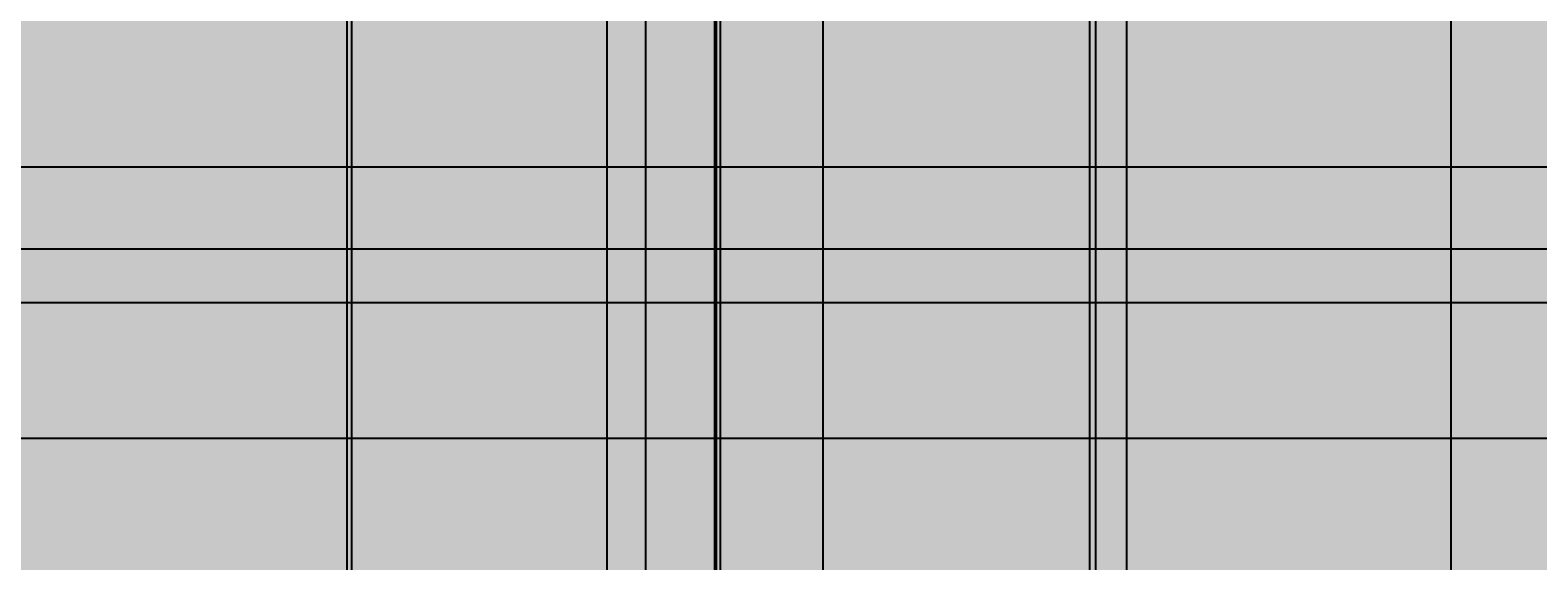
# Model space of a CAD drawing. Units: inches. Extents: x 818 to 1898, y 976 to 2364.
# Tile 75 of 96: x 1260 to 1372, y 2054 to 2093. Entities that reach past the tile are written whole.
import ezdxf

# ---------------------------------------------------------------- set-up
doc = ezdxf.new("R2010")
doc.units = ezdxf.units.IN
doc.header["$LTSCALE"] = 5
doc.header["$MEASUREMENT"] = 0
doc.layers.add('A-ANNO-DIMS', color=2, linetype='Continuous', lineweight=18)
doc.layers.add('L-PLNT-PATT', color=114, linetype='Continuous', lineweight=9, true_color=0x139b48)
doc.styles.get("Standard").update_dxf_attribs({"font": 'arial.ttf'})
doc.dimstyles.get("Standard").update_dxf_attribs({"dimtxt": 0.18, "dimasz": 0.18, "dimexe": 0.18, "dimexo": 0.0625, "dimgap": 0.09, "dimtad": 0, "dimtih": 1, "dimtoh": 1, "dimdec": 4, "dimzin": 0, "dimdsep": 46, "dimtxsty": 'Standard', "dimcen": 0.09, "dimadec": 0, "dimazin": 0, "dimtfac": 1, "dimtdec": 4, "dimtofl": 0, "dimtmove": 0, "dimatfit": 3, "dimfxl": 1, "dimtolj": 1, "dimtzin": 0, "dimarcsym": 0})

# ---------------------------------------------------------------- blocks, each defined once
blk = doc.blocks.new('*D61')
at = {"layer": 'A-ANNO-DIMS', "color": 0, "lineweight": -2, "ltscale": 5, "transparency": 16777216}
for p, q in [((1071.73, 1203.03), (1071.73, 2363.87)), ((1071.91, 2363.69), (1250.94, 2363.69)), ((1430.55, 2363.69), (1251.51, 2363.69)), ((1430.73, 1203.03), (1430.73, 2363.87))]:
    blk.add_line(p, q, dxfattribs=at)
at = {"layer": 'A-ANNO-DIMS', "color": 0, "ltscale": 5, "transparency": 16777216}
for points in [[(1071.91, 2363.72), (1071.91, 2363.66), (1071.73, 2363.69)], [(1430.55, 2363.72), (1430.55, 2363.66), (1430.73, 2363.69)]]:
    blk.add_solid(points, dxfattribs=at)
at = {"layer": 'Defpoints', "color": 0, "ltscale": 5, "transparency": 16777216}
for p in [(1430.73, 2363.69), (1071.73, 1202.96), (1430.73, 1202.96)]:
    blk.add_point(p, dxfattribs=at)
at = {"layer": 'A-ANNO-DIMS', "color": 0, "ltscale": 5, "transparency": 16777216, "insert": (1251.23, 2363.69), "char_height": 0.18, "attachment_point": 5}
blk.add_mtext('\\A1;359', dxfattribs=at)
blk = doc.blocks.new('*D64')
at = {"layer": 'A-ANNO-DIMS', "color": 0, "lineweight": -2, "ltscale": 5, "transparency": 16777216}
for p, q in [((1197.73, 1501.14), (1197.73, 2363.87)), ((1197.91, 2363.69), (1313.93, 2363.69)), ((1430.55, 2363.69), (1314.52, 2363.69)), ((1430.73, 1501.14), (1430.73, 2363.87))]:
    blk.add_line(p, q, dxfattribs=at)
at = {"layer": 'A-ANNO-DIMS', "color": 0, "ltscale": 5, "transparency": 16777216}
for points in [[(1197.91, 2363.72), (1197.91, 2363.66), (1197.73, 2363.69)], [(1430.55, 2363.72), (1430.55, 2363.66), (1430.73, 2363.69)]]:
    blk.add_solid(points, dxfattribs=at)
at = {"layer": 'Defpoints', "color": 0, "ltscale": 5, "transparency": 16777216}
for p in [(1430.73, 2363.69), (1197.73, 1501.08), (1430.73, 1501.08)]:
    blk.add_point(p, dxfattribs=at)
at = {"layer": 'A-ANNO-DIMS', "color": 0, "ltscale": 5, "transparency": 16777216, "insert": (1314.23, 2363.69), "char_height": 0.18, "attachment_point": 5}
blk.add_mtext('\\A1;233', dxfattribs=at)
blk = doc.blocks.new('*D86')
at = {"layer": 'A-ANNO-DIMS', "color": 0, "lineweight": -2, "ltscale": 5, "transparency": 16777216}
for p, q in [((1258.73, 2053.14), (1258.73, 2363.87)), ((1258.91, 2363.69), (1486.43, 2363.69)), ((1714.55, 2363.69), (1487.02, 2363.69)), ((1714.73, 2053.14), (1714.73, 2363.87))]:
    blk.add_line(p, q, dxfattribs=at)
at = {"layer": 'A-ANNO-DIMS', "color": 0, "ltscale": 5, "transparency": 16777216}
for points in [[(1258.91, 2363.72), (1258.91, 2363.66), (1258.73, 2363.69)], [(1714.55, 2363.72), (1714.55, 2363.66), (1714.73, 2363.69)]]:
    blk.add_solid(points, dxfattribs=at)
at = {"layer": 'Defpoints', "color": 0, "ltscale": 5, "transparency": 16777216}
for p in [(1714.73, 2363.69), (1258.73, 2053.08), (1714.73, 2053.08)]:
    blk.add_point(p, dxfattribs=at)
at = {"layer": 'A-ANNO-DIMS', "color": 0, "ltscale": 5, "transparency": 16777216, "insert": (1486.73, 2363.69), "char_height": 0.18, "attachment_point": 5}
blk.add_mtext('\\A1;456', dxfattribs=at)
blk = doc.blocks.new('*D96')
at = {"layer": 'A-ANNO-DIMS', "color": 0, "lineweight": -2, "ltscale": 5, "transparency": 16777216}
for p, q in [((1229.65, 1071.12), (1229.65, 2363.87)), ((1229.83, 2363.69), (1256.52, 2363.69)), ((1283.99, 2363.69), (1257.3, 2363.69)), ((1284.17, 1071.12), (1284.17, 2363.87))]:
    blk.add_line(p, q, dxfattribs=at)
at = {"layer": 'A-ANNO-DIMS', "color": 0, "ltscale": 5, "transparency": 16777216}
for points in [[(1229.83, 2363.72), (1229.83, 2363.66), (1229.65, 2363.69)], [(1283.99, 2363.72), (1283.99, 2363.66), (1284.17, 2363.69)]]:
    blk.add_solid(points, dxfattribs=at)
at = {"layer": 'Defpoints', "color": 0, "ltscale": 5, "transparency": 16777216}
for p in [(1284.17, 2363.69), (1229.65, 1071.06), (1284.17, 1071.06)]:
    blk.add_point(p, dxfattribs=at)
at = {"layer": 'A-ANNO-DIMS', "color": 0, "ltscale": 5, "transparency": 16777216, "insert": (1256.91, 2363.69), "char_height": 0.18, "attachment_point": 5}
blk.add_mtext('\\A1;54.52', dxfattribs=at)
blk = doc.blocks.new('*D97')
at = {"layer": 'A-ANNO-DIMS', "color": 0, "lineweight": -2, "ltscale": 5, "transparency": 16777216}
for p, q in [((1284.17, 1071.12), (1284.17, 2363.87)), ((1284.35, 2363.69), (1310.96, 2363.69)), ((1338.36, 2363.69), (1311.75, 2363.69)), ((1338.54, 1071.12), (1338.54, 2363.87))]:
    blk.add_line(p, q, dxfattribs=at)
at = {"layer": 'A-ANNO-DIMS', "color": 0, "ltscale": 5, "transparency": 16777216}
for points in [[(1284.35, 2363.72), (1284.35, 2363.66), (1284.17, 2363.69)], [(1338.36, 2363.72), (1338.36, 2363.66), (1338.54, 2363.69)]]:
    blk.add_solid(points, dxfattribs=at)
at = {"layer": 'Defpoints', "color": 0, "ltscale": 5, "transparency": 16777216}
for p in [(1338.54, 2363.69), (1284.17, 1071.06), (1338.54, 1071.06)]:
    blk.add_point(p, dxfattribs=at)
at = {"layer": 'A-ANNO-DIMS', "color": 0, "ltscale": 5, "transparency": 16777216, "insert": (1311.36, 2363.69), "char_height": 0.18, "attachment_point": 5}
blk.add_mtext('\\A1;54.37', dxfattribs=at)
blk = doc.blocks.new('*D98')
at = {"layer": 'A-ANNO-DIMS', "color": 0, "lineweight": -2, "ltscale": 5, "transparency": 16777216}
for p, q in [((1338.54, 1071.12), (1338.54, 2363.87)), ((1338.72, 2363.69), (1364.81, 2363.69)), ((1391.7, 2363.69), (1365.6, 2363.69)), ((1391.88, 1071.12), (1391.88, 2363.87))]:
    blk.add_line(p, q, dxfattribs=at)
at = {"layer": 'A-ANNO-DIMS', "color": 0, "ltscale": 5, "transparency": 16777216}
for points in [[(1338.72, 2363.72), (1338.72, 2363.66), (1338.54, 2363.69)], [(1391.7, 2363.72), (1391.7, 2363.66), (1391.88, 2363.69)]]:
    blk.add_solid(points, dxfattribs=at)
at = {"layer": 'Defpoints', "color": 0, "ltscale": 5, "transparency": 16777216}
for p in [(1391.88, 2363.69), (1338.54, 1071.06), (1391.88, 1071.06)]:
    blk.add_point(p, dxfattribs=at)
at = {"layer": 'A-ANNO-DIMS', "color": 0, "ltscale": 5, "transparency": 16777216, "insert": (1365.21, 2363.69), "char_height": 0.18, "attachment_point": 5}
blk.add_mtext('\\A1;53.33', dxfattribs=at)
blk = doc.blocks.new('*D141')
at = {"layer": 'A-ANNO-DIMS', "color": 0, "lineweight": -2, "ltscale": 5, "transparency": 16777216}
for p, q in [((1218.17, 2083.26), (1897.92, 2083.26)), ((1897.74, 2083.08), (1897.74, 2073.44)), ((1897.74, 2063.44), (1897.74, 2073.08)), ((1198.17, 2063.26), (1897.92, 2063.26))]:
    blk.add_line(p, q, dxfattribs=at)
at = {"layer": 'A-ANNO-DIMS', "color": 0, "ltscale": 5, "transparency": 16777216}
for points in [[(1897.71, 2083.08), (1897.77, 2083.08), (1897.74, 2083.26)], [(1897.71, 2063.44), (1897.77, 2063.44), (1897.74, 2063.26)]]:
    blk.add_solid(points, dxfattribs=at)
at = {"layer": 'Defpoints', "color": 0, "ltscale": 5, "transparency": 16777216}
for p in [(1218.11, 2083.26), (1198.11, 2063.26), (1897.74, 2063.26)]:
    blk.add_point(p, dxfattribs=at)
at = {"layer": 'A-ANNO-DIMS', "color": 0, "ltscale": 5, "transparency": 16777216, "insert": (1897.74, 2073.26), "char_height": 0.18, "attachment_point": 5}
blk.add_mtext('\\A1;20', dxfattribs=at)
blk = doc.blocks.new('*D142')
at = {"layer": 'A-ANNO-DIMS', "color": 0, "lineweight": -2, "ltscale": 5, "transparency": 16777216}
for p, q in [((1208.17, 2073.26), (1897.92, 2073.26)), ((1897.74, 2073.08), (1897.74, 2068.44)), ((1897.74, 2063.44), (1897.74, 2068.08)), ((1198.17, 2063.26), (1897.92, 2063.26))]:
    blk.add_line(p, q, dxfattribs=at)
at = {"layer": 'A-ANNO-DIMS', "color": 0, "ltscale": 5, "transparency": 16777216}
for points in [[(1897.71, 2073.08), (1897.77, 2073.08), (1897.74, 2073.26)], [(1897.71, 2063.44), (1897.77, 2063.44), (1897.74, 2063.26)]]:
    blk.add_solid(points, dxfattribs=at)
at = {"layer": 'Defpoints', "color": 0, "ltscale": 5, "transparency": 16777216}
for p in [(1208.11, 2073.26), (1897.74, 2073.26), (1198.11, 2063.26)]:
    blk.add_point(p, dxfattribs=at)
at = {"layer": 'A-ANNO-DIMS', "color": 0, "ltscale": 5, "transparency": 16777216, "insert": (1897.74, 2068.26), "char_height": 0.18, "attachment_point": 5}
blk.add_mtext('\\A1;10', dxfattribs=at)
blk = doc.blocks.new('*D165')
at = {"layer": 'A-ANNO-DIMS', "color": 0, "lineweight": -2, "ltscale": 5, "transparency": 16777216}
for p, q in [((1283.82, 1510.14), (1283.82, 2363.87)), ((1284, 2363.69), (1324.09, 2363.69)), ((1364.97, 2363.69), (1324.88, 2363.69)), ((1365.15, 1510.14), (1365.15, 2363.87))]:
    blk.add_line(p, q, dxfattribs=at)
at = {"layer": 'A-ANNO-DIMS', "color": 0, "ltscale": 5, "transparency": 16777216}
for points in [[(1284, 2363.72), (1284, 2363.66), (1283.82, 2363.69)], [(1364.97, 2363.72), (1364.97, 2363.66), (1365.15, 2363.69)]]:
    blk.add_solid(points, dxfattribs=at)
at = {"layer": 'Defpoints', "color": 0, "ltscale": 5, "transparency": 16777216}
for p in [(1365.15, 2363.69), (1283.82, 1510.08), (1365.15, 1510.08)]:
    blk.add_point(p, dxfattribs=at)
at = {"layer": 'A-ANNO-DIMS', "color": 0, "ltscale": 5, "transparency": 16777216, "insert": (1324.48, 2363.69), "char_height": 0.18, "attachment_point": 5}
blk.add_mtext('\\A1;81.33', dxfattribs=at)
blk = doc.blocks.new('*D235')
at = {"layer": 'A-ANNO-DIMS', "color": 0, "lineweight": -2, "ltscale": 5, "transparency": 16777216}
for p, q in [((1310.91, 2026.27), (1310.91, 2363.87)), ((1311.09, 2363.69), (1324.48, 2363.69)), ((1338.81, 2363.69), (1325.41, 2363.69)), ((1338.99, 2026.27), (1338.99, 2363.87))]:
    blk.add_line(p, q, dxfattribs=at)
at = {"layer": 'A-ANNO-DIMS', "color": 0, "ltscale": 5, "transparency": 16777216}
for points in [[(1311.09, 2363.72), (1311.09, 2363.66), (1310.91, 2363.69)], [(1338.81, 2363.72), (1338.81, 2363.66), (1338.99, 2363.69)]]:
    blk.add_solid(points, dxfattribs=at)
at = {"layer": 'Defpoints', "color": 0, "ltscale": 5, "transparency": 16777216}
for p in [(1338.99, 2363.69), (1310.91, 2026.21), (1338.99, 2026.21)]:
    blk.add_point(p, dxfattribs=at)
at = {"layer": 'A-ANNO-DIMS', "color": 0, "ltscale": 5, "transparency": 16777216, "insert": (1324.95, 2363.69), "char_height": 0.18, "attachment_point": 5}
blk.add_mtext('\\A1;28.084', dxfattribs=at)
blk = doc.blocks.new('*D257')
at = {"layer": 'A-ANNO-DIMS', "color": 0, "lineweight": -2, "ltscale": 5, "transparency": 16777216}
for p, q in [((1399.57, 2077.19), (818.03, 2077.19)), ((818.21, 2077.01), (818.21, 2065.31)), ((818.21, 2053.26), (818.21, 2064.95)), ((1399.57, 2053.08), (818.03, 2053.08))]:
    blk.add_line(p, q, dxfattribs=at)
at = {"layer": 'A-ANNO-DIMS', "color": 0, "ltscale": 5, "transparency": 16777216}
for points in [[(818.18, 2077.01), (818.24, 2077.01), (818.21, 2077.19)], [(818.18, 2053.26), (818.24, 2053.26), (818.21, 2053.08)]]:
    blk.add_solid(points, dxfattribs=at)
at = {"layer": 'Defpoints', "color": 0, "ltscale": 5, "transparency": 16777216}
for p in [(818.21, 2077.19), (1399.64, 2077.19), (1399.64, 2053.08)]:
    blk.add_point(p, dxfattribs=at)
at = {"layer": 'A-ANNO-DIMS', "color": 0, "ltscale": 5, "transparency": 16777216, "insert": (818.21, 2065.13), "char_height": 0.18, "attachment_point": 5}
blk.add_mtext('\\A1;24.11', dxfattribs=at)
blk = doc.blocks.new('*D269')
at = {"layer": 'A-ANNO-DIMS', "color": 0, "lineweight": -2, "ltscale": 5, "transparency": 16777216}
for p, q in [((1246.94, 1534.14), (1246.94, 2363.87)), ((1247.12, 2363.69), (1293.71, 2363.69)), ((1341.08, 2363.69), (1294.49, 2363.69)), ((1341.26, 1534.14), (1341.26, 2363.87))]:
    blk.add_line(p, q, dxfattribs=at)
at = {"layer": 'A-ANNO-DIMS', "color": 0, "ltscale": 5, "transparency": 16777216}
for points in [[(1247.12, 2363.72), (1247.12, 2363.66), (1246.94, 2363.69)], [(1341.08, 2363.72), (1341.08, 2363.66), (1341.26, 2363.69)]]:
    blk.add_solid(points, dxfattribs=at)
at = {"layer": 'Defpoints', "color": 0, "ltscale": 5, "transparency": 16777216}
for p in [(1341.26, 2363.69), (1246.94, 1534.08), (1341.26, 1534.08)]:
    blk.add_point(p, dxfattribs=at)
at = {"layer": 'A-ANNO-DIMS', "color": 0, "ltscale": 5, "transparency": 16777216, "insert": (1294.1, 2363.69), "char_height": 0.18, "attachment_point": 5}
blk.add_mtext('\\A1;94.32', dxfattribs=at)
blk = doc.blocks.new('*D274')
at = {"layer": 'A-ANNO-DIMS', "color": 0, "lineweight": -2, "ltscale": 5, "transparency": 16777216}
for p, q in [((1311.03, 1897.93), (1311.03, 2363.87)), ((1311.21, 2363.69), (1344.01, 2363.69)), ((1377.6, 2363.69), (1344.8, 2363.69)), ((1377.78, 1897.93), (1377.78, 2363.87))]:
    blk.add_line(p, q, dxfattribs=at)
at = {"layer": 'A-ANNO-DIMS', "color": 0, "ltscale": 5, "transparency": 16777216}
for points in [[(1311.21, 2363.72), (1311.21, 2363.66), (1311.03, 2363.69)], [(1377.6, 2363.72), (1377.6, 2363.66), (1377.78, 2363.69)]]:
    blk.add_solid(points, dxfattribs=at)
at = {"layer": 'Defpoints', "color": 0, "ltscale": 5, "transparency": 16777216}
for p in [(1377.78, 2363.69), (1311.03, 1897.87), (1377.78, 1897.87)]:
    blk.add_point(p, dxfattribs=at)
at = {"layer": 'A-ANNO-DIMS', "color": 0, "ltscale": 5, "transparency": 16777216, "insert": (1344.4, 2363.69), "char_height": 0.18, "attachment_point": 5}
blk.add_mtext('\\A1;66.75', dxfattribs=at)
blk = doc.blocks.new('*D281')
at = {"layer": 'A-ANNO-DIMS', "color": 0, "lineweight": -2, "ltscale": 5, "transparency": 16777216}
for p, q in [((1250.3, 1913.7), (1250.3, 2363.87)), ((1250.48, 2363.69), (1420.12, 2363.69)), ((1590.55, 2363.69), (1420.91, 2363.69)), ((1590.73, 2011.14), (1590.73, 2363.87))]:
    blk.add_line(p, q, dxfattribs=at)
at = {"layer": 'A-ANNO-DIMS', "color": 0, "ltscale": 5, "transparency": 16777216}
for points in [[(1250.48, 2363.72), (1250.48, 2363.66), (1250.3, 2363.69)], [(1590.55, 2363.72), (1590.55, 2363.66), (1590.73, 2363.69)]]:
    blk.add_solid(points, dxfattribs=at)
at = {"layer": 'Defpoints', "color": 0, "ltscale": 5, "transparency": 16777216}
for p in [(1590.73, 2363.69), (1590.73, 2011.08), (1250.3, 1913.64)]:
    blk.add_point(p, dxfattribs=at)
at = {"layer": 'A-ANNO-DIMS', "color": 0, "ltscale": 5, "transparency": 16777216, "insert": (1420.51, 2363.69), "char_height": 0.18, "attachment_point": 5}
blk.add_mtext('\\A1;340.4', dxfattribs=at)
blk = doc.blocks.new('*D286')
at = {"layer": 'A-ANNO-DIMS', "color": 0, "lineweight": -2, "ltscale": 5, "transparency": 16777216}
for p, q in [((1305.83, 1851.97), (1305.83, 2363.87)), ((1306.01, 2363.69), (1308.18, 2363.69)), ((1311.15, 2363.69), (1308.97, 2363.69)), ((1311.33, 1853.81), (1311.33, 2363.87))]:
    blk.add_line(p, q, dxfattribs=at)
at = {"layer": 'A-ANNO-DIMS', "color": 0, "ltscale": 5, "transparency": 16777216}
for points in [[(1306.01, 2363.72), (1306.01, 2363.66), (1305.83, 2363.69)], [(1311.15, 2363.72), (1311.15, 2363.66), (1311.33, 2363.69)]]:
    blk.add_solid(points, dxfattribs=at)
at = {"layer": 'Defpoints', "color": 0, "ltscale": 5, "transparency": 16777216}
for p in [(1305.83, 2363.69), (1311.33, 1853.75), (1305.83, 1851.91)]:
    blk.add_point(p, dxfattribs=at)
at = {"layer": 'A-ANNO-DIMS', "color": 0, "ltscale": 5, "transparency": 16777216, "insert": (1308.58, 2363.69), "char_height": 0.18, "attachment_point": 5}
blk.add_mtext('\\A1;5.499', dxfattribs=at)
blk = doc.blocks.new('*D290')
at = {"layer": 'A-ANNO-DIMS', "color": 0, "lineweight": -2, "ltscale": 5, "transparency": 16777216}
for p, q in [((1302.98, 1599.43), (1302.98, 2363.87)), ((1303.16, 2363.69), (1310.57, 2363.69)), ((1318.71, 2363.69), (1311.31, 2363.69)), ((1318.89, 1607.83), (1318.89, 2363.87))]:
    blk.add_line(p, q, dxfattribs=at)
at = {"layer": 'A-ANNO-DIMS', "color": 0, "ltscale": 5, "transparency": 16777216}
for points in [[(1303.16, 2363.72), (1303.16, 2363.66), (1302.98, 2363.69)], [(1318.71, 2363.72), (1318.71, 2363.66), (1318.89, 2363.69)]]:
    blk.add_solid(points, dxfattribs=at)
at = {"layer": 'Defpoints', "color": 0, "ltscale": 5, "transparency": 16777216}
for p in [(1318.89, 2363.69), (1318.89, 1607.77), (1302.98, 1599.37)]:
    blk.add_point(p, dxfattribs=at)
at = {"layer": 'A-ANNO-DIMS', "color": 0, "ltscale": 5, "transparency": 16777216, "insert": (1310.94, 2363.69), "char_height": 0.18, "attachment_point": 5}
blk.add_mtext('\\A1;15.91', dxfattribs=at)

msp = doc.modelspace()

# ---------------------------------------------------------------- hatches: boundary and pattern name
at = {"layer": 'L-PLNT-PATT', "ltscale": 5}
h = msp.add_hatch(color=256, dxfattribs=at)
h.dxf.hatch_style = 1
h.paths.add_polyline_path([(1789.7173, 2205.9709), (1083.7252, 2205.9709), (1083.7252, 2083.2623), (1218.1114, 2083.2623), (1218.1114, 2053.0782), (1390.6356, 2053.0782), (1390.6356, 2081.1881), (1399.6356, 2081.1881), (1413.02, 2081.1881), (1422.02, 2081.1881), (1422.02, 2053.0782), (1676.6446, 2053.0782), (1676.6446, 2081.1881), (1714.7251, 2081.1881), (1714.7251, 2081.6235), (1789.7173, 2081.6235)])
h.paths.add_polyline_path([(1388.6037, 2145.2461), (1388.6037, 2122.3767), (1373.4756, 2122.3767), (1373.4756, 2145.2461)], flags=16)
h.paths.add_polyline_path([(1408.6922, 2145.2461), (1423.8203, 2145.2461), (1423.8203, 2122.3767), (1408.6922, 2122.3767)], flags=16)
h.paths.add_polyline_path([(1353.3871, 2155.7839), (1353.3871, 2122.3767), (1338.259, 2122.3767), (1338.259, 2155.7839)], flags=16)
h.paths.add_polyline_path([(1443.9089, 2158.4222), (1459.037, 2158.4222), (1459.037, 2122.3767), (1443.9089, 2122.3767)], flags=16)
h.paths.add_polyline_path([(1318.1705, 2145.2461), (1318.1705, 2122.3767), (1303.0424, 2122.3767), (1303.0424, 2145.2461)], flags=16)
h.paths.add_polyline_path([(1479.1255, 2145.2461), (1494.2536, 2145.2461), (1494.2536, 2122.3767), (1479.1255, 2122.3767)], flags=16)
h.paths.add_polyline_path([(1282.9539, 2145.2461), (1282.9539, 2122.3767), (1267.8258, 2122.3767), (1267.8258, 2145.2461)], flags=16)
h.paths.add_polyline_path([(1514.3421, 2145.2461), (1529.4702, 2145.2461), (1529.4702, 2122.3767), (1514.3421, 2122.3767)], flags=16)
h.paths.add_polyline_path([(1247.7373, 2159.4296), (1247.7373, 2122.3767), (1232.6091, 2122.3767), (1232.6091, 2159.4296)], flags=16)
h.paths.add_polyline_path([(1549.5587, 2156.9246), (1564.6868, 2156.9246), (1564.6868, 2122.3767), (1549.5587, 2122.3767)], flags=16)
h.paths.add_polyline_path([(1212.5206, 2145.2461), (1212.5206, 2122.3767), (1197.3925, 2122.3767), (1197.3925, 2145.2461)], flags=16)
h.paths.add_polyline_path([(1584.7753, 2145.2461), (1599.9034, 2145.2461), (1599.9034, 2122.3767), (1584.7753, 2122.3767)], flags=16)
h.paths.add_polyline_path([(1185.1073, 2104.7786), (1190.6407, 2104.7786), (1185.1073, 2098.2505), (1179.5738, 2104.7786)], flags=16)
h.paths.add_polyline_path([(1619.9919, 2145.2461), (1635.1201, 2145.2461), (1635.1201, 2122.3767), (1619.9919, 2122.3767)], flags=16)
h.paths.add_polyline_path([(1655.2086, 2156.1761), (1670.3367, 2156.1761), (1670.3367, 2122.3767), (1655.2086, 2122.3767)], flags=16)
h.paths.add_polyline_path([(1686.5992, 2145.2461), (1701.7273, 2145.2461), (1701.7273, 2122.3767), (1686.5992, 2122.3767)], flags=16)
h.paths.add_polyline_path([(1715.7616, 2145.2461), (1730.8897, 2145.2461), (1730.8897, 2122.3767), (1715.7616, 2122.3767)], flags=16)
h.paths.add_polyline_path([(1753.1652, 2145.2461), (1776.3312, 2145.2461), (1776.3312, 2115.6891), (1753.1652, 2115.6891)], flags=16)
h.paths.add_polyline_path([(1191.4331, 2146.5159), (1176.7891, 2146.5159), (1176.7891, 2134.1516), (1191.4331, 2134.1516)], flags=24)

# ---------------------------------------------------------------- dimensions: what is measured, and where the dimension line sits
at = {"layer": 'A-ANNO-DIMS', "ltscale": 5}
for base, p1, p2, override, picture, middle in [((1430.7251, 2363.6929), (1071.7251, 1202.9642), (1430.7251, 1202.9642), {"dimdec": 0, "dimlfac": 1, "dimrnd": 0, "dimzin": 0, "dimdsep": 46, "dimlunit": 2}, '*D61', (1251.2251, 2363.6929)), ((1430.7251, 2363.6929), (1197.7251, 1501.0782), (1430.7251, 1501.0782), {"dimdec": 0, "dimlfac": 1, "dimrnd": 0, "dimzin": 0, "dimdsep": 46, "dimlunit": 2}, '*D64', (1314.2251, 2363.6929)), ((1284.1697, 2363.6929), (1229.6474, 1071.0552), (1284.1697, 1071.0552), {"dimdec": 2, "dimlfac": 1, "dimrnd": 0, "dimzin": 0, "dimdsep": 46, "dimlunit": 2}, '*D96', (1256.9085, 2363.6929)), ((1341.2593, 2363.6929), (1246.9377, 1534.0782), (1341.2593, 1534.0782), {"dimdec": 2, "dimlfac": 1, "dimrnd": 0, "dimzin": 0, "dimdsep": 46, "dimlunit": 2}, '*D269', (1294.0985, 2363.6929)), ((1590.7251, 2363.6929), (1250.3029, 1913.6401), (1590.7251, 2011.0782), {"dimdec": 1, "dimlfac": 1, "dimrnd": 0, "dimzin": 0, "dimdsep": 46, "dimlunit": 2}, '*D281', (1420.514, 2363.6929)), ((1714.7251, 2363.6929), (1258.7251, 2053.0782), (1714.7251, 2053.0782), {"dimdec": 0, "dimlfac": 1, "dimrnd": 0, "dimzin": 0, "dimdsep": 46, "dimlunit": 2}, '*D86', (1486.7251, 2363.6929)), ((1365.1463, 2363.6929), (1283.8183, 1510.0782), (1365.1463, 1510.0782), {"dimdec": 2, "dimlfac": 1, "dimrnd": 0, "dimzin": 0, "dimdsep": 46, "dimlunit": 2}, '*D165', (1324.4823, 2363.6929)), ((1338.5412, 2363.6929), (1284.1697, 1071.0552), (1338.5412, 1071.0552), {"dimdec": 2, "dimlfac": 1, "dimrnd": 0, "dimzin": 0, "dimdsep": 46, "dimlunit": 2}, '*D97', (1311.3554, 2363.6929)), ((1318.8931, 2363.6929), (1302.9835, 1599.3725), (1318.8931, 1607.7707), {"dimdec": 2, "dimlfac": 1, "dimrnd": 0, "dimzin": 0, "dimdsep": 46, "dimlunit": 2}, '*D290', (1310.9383, 2363.6929)), ((1305.8278, 2363.6929), (1311.3271, 1853.7496), (1305.8278, 1851.9081), {"dimdec": 3, "dimlfac": 1, "dimrnd": 0, "dimzin": 0, "dimdsep": 46, "dimlunit": 2}, '*D286', (1308.5774, 2363.6929)), ((1338.9915, 2363.6929), (1310.9077, 2026.2074), (1338.9915, 2026.2074), {"dimdec": 3, "dimlfac": 1, "dimrnd": 0, "dimzin": 0, "dimdsep": 46, "dimlunit": 2}, '*D235', (1324.9496, 2363.6929)), ((1377.7791, 2363.6929), (1311.025, 1897.8663), (1377.7791, 1897.8663), {"dimdec": 2, "dimlfac": 1, "dimrnd": 0, "dimzin": 0, "dimdsep": 46, "dimlunit": 2}, '*D274', (1344.4021, 2363.6929)), ((1391.8757, 2363.6929), (1338.5412, 1071.0552), (1391.8757, 1071.0552), {"dimdec": 2, "dimlfac": 1, "dimrnd": 0, "dimzin": 0, "dimdsep": 46, "dimlunit": 2}, '*D98', (1365.2084, 2363.6929))]:
    dim = msp.add_linear_dim(base=base, p1=p1, p2=p2, dimstyle='Standard', override=override, dxfattribs=at)
    dim.commit()
    dim.dimension.update_dxf_attribs({"geometry": picture, "text_midpoint": middle})
for base, p1, p2, override, picture, middle in [((1897.736, 2063.2623), (1218.1114, 2083.2623), (1198.1114, 2063.2623), {"dimdec": 0, "dimlfac": 1, "dimrnd": 0, "dimzin": 0, "dimdsep": 46, "dimlunit": 2}, '*D141', (1897.736, 2073.2623)), ((818.2059, 2077.1881), (1399.6356, 2053.0782), (1399.6356, 2077.1881), {"dimdec": 2, "dimlfac": 1, "dimrnd": 0, "dimzin": 0, "dimdsep": 46, "dimlunit": 2}, '*D257', (818.2059, 2065.1332)), ((1897.736, 2073.2623), (1198.1114, 2063.2623), (1208.1114, 2073.2623), {"dimdec": 0, "dimlfac": 1, "dimrnd": 0, "dimzin": 0, "dimdsep": 46, "dimlunit": 2}, '*D142', (1897.736, 2068.2623))]:
    dim = msp.add_linear_dim(base=base, p1=p1, p2=p2, angle=90, dimstyle='Standard', override=override, dxfattribs=at)
    dim.commit()
    dim.dimension.update_dxf_attribs({"geometry": picture, "text_midpoint": middle})

doc.saveas('drawing.dxf')
